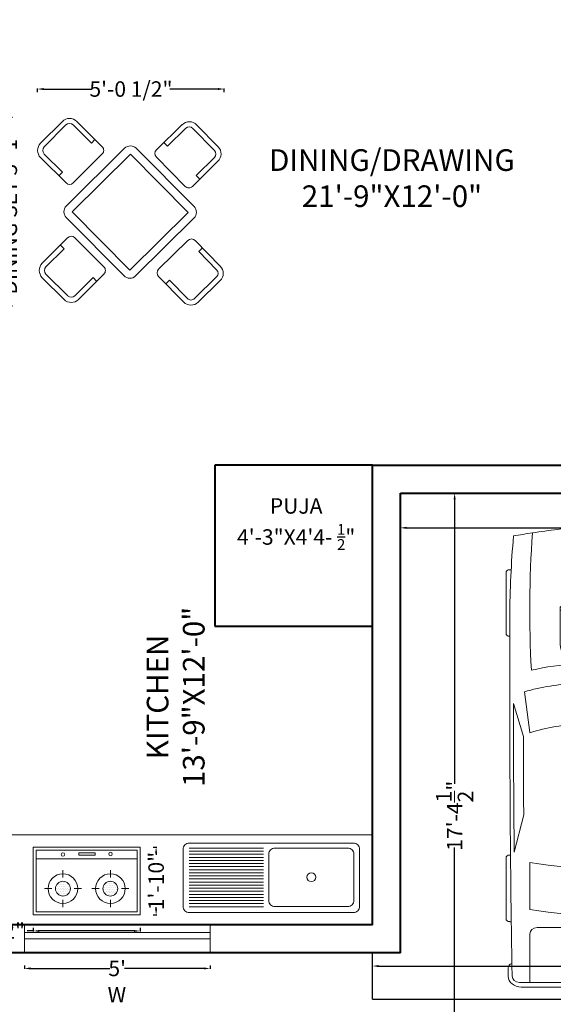
# Model space of a CAD drawing. Units: inches. Extents: x -231 to 349, y -511 to 252.
# Tile 3 of 6: x -36 to 136, y -351 to -33. Entities that reach past the tile are written whole.
import ezdxf

# ---------------------------------------------------------------- set-up
doc = ezdxf.new("R2010")
doc.units = ezdxf.units.IN
doc.header["$MEASUREMENT"] = 0
for name, color, linetype, lineweight in [('A-ANNO-DIMS', 7, 'Continuous', 18), ('A-ANNO-TEXT', 7, 'Continuous', 18), ('A-AREA-IDEN', 7, 'Continuous', 25), ('A-EQPM', 8, 'Continuous', 18), ('A-FLOR', 7, 'Continuous', 25), ('A-FLOR-CASE', 30, 'Continuous', 20), ('A-FLOR-FIXT', 8, 'Continuous', 18), ('A-FLOR-FIXT-PATT', 8, 'Continuous', 13), ('A-FURN', 8, 'Continuous', 18), ('A-GLAZ', 177, 'Continuous', 20), ('A-WALL', 7, 'Continuous', 40), ('C-PARK-VEHI', 8, 'Continuous', 13)]:
    doc.layers.add(name, color=color, linetype=linetype, lineweight=lineweight)
doc.styles.get("Standard").update_dxf_attribs({"font": 'arial.ttf'})
doc.dimstyles.get("Standard").update_dxf_attribs({"dimtxt": 5, "dimasz": 2, "dimexe": 0.18, "dimexo": 0.0625, "dimgap": 0.09, "dimtad": 0, "dimzin": 0, "dimdsep": 46, "dimlunit": 4, "dimtxsty": 'Standard', "dimcen": 0.09, "dimadec": 0, "dimazin": 0, "dimtfac": 1, "dimtofl": 0, "dimtmove": 0, "dimatfit": 3, "dimfxl": 1, "dimfxlon": 1, "dimtolj": 1, "dimtzin": 0, "dimarcsym": 0})

# ---------------------------------------------------------------- blocks, each defined once
blk = doc.blocks.new('*U7')
for p, q in [((21.1, 37.41), (21.1, 36.83)), ((46.55, 38.89), (22.35, 38.89)), ((47.8, 37.39), (47.8, 37.41)), ((87.99, 31.87), (74.76, 35.92)), ((134.31, 35.6), (119.29, 31.78)), ((135.45, 37.07), (135.45, 37.41)), ((136.7, 38.89), (160.9, 38.89)), ((162.15, 37.41), (162.15, 36.77)), ((186.47, -33.5), (186.47, 33.5)), ((188.4, -32.76), (188.4, 32.76)), ((70.03, 31.54), (86.41, 29.35)), ((138.42, 29.35), (157.25, 29.35)), ((186.47, 29.35), (167.01, 29.35)), ((164.52, 26.39), (164.52, -26.39)), ((32.27, 11.63), (36.13, 17.17)), ((36.13, 17.17), (50.94, 17.17)), ((29.77, 9.51), (51.68, 9.51)), ((32.12, 9.51), (32.12, 11.15)), ((58.92, -10.77), (58.92, 10.77)), ((66.55, -10.53), (66.55, 10.53)), ((82.74, 8.5), (82.74, -8.5)), ((186.47, -10.53), (186.47, 10.53)), ((3.27, 6.13), (0.1, 0.41)), ((0, 0), (51.68, 0)), ((0.1, -0.41), (3.27, -6.13)), ((29.77, -9.51), (51.68, -9.51)), ((32.12, -9.51), (32.12, -11.15)), ((32.27, -11.63), (36.13, -17.17)), ((36.13, -17.17), (50.94, -17.17)), ((86.41, -29.35), (70.03, -31.54)), ((157.25, -29.35), (138.42, -29.35)), ((167.01, -29.35), (186.47, -29.35)), ((87.99, -31.87), (74.76, -35.92)), ((134.31, -35.6), (119.29, -31.78)), ((21.1, -37.41), (21.1, -36.83)), ((46.55, -38.89), (22.35, -38.89)), ((47.8, -37.39), (47.8, -37.41)), ((135.45, -37.07), (135.45, -37.41)), ((136.7, -38.89), (160.9, -38.89)), ((162.15, -37.41), (162.15, -36.77))]:
    blk.add_line(p, q)
for centre, major_axis, ratio, start_param, end_param in [((266.03, -27.52), (0, 313.31), 0.842304, 1.367076, 1.39176), ((41.19, -490.86), (0, 528.23), 0.842304, 0.00281, 0.075598), ((22.35, 37.41), (0, -1.48), 0.842304, 3.141593, 4.712389), ((64.48, -10555.62), (0, 10593.03), 0.842304, -0.013397, 0.002797), ((46.55, 37.41), (0, 1.48), 0.842304, -1.570796, 0), ((64.48, -10555.62), (0, -10591.55), 0.842304, 3.133765, 3.140441), ((136.7, 37.41), (0, -1.48), 0.842304, 3.141593, 4.712389), ((160.9, 37.41), (0, 1.48), 0.842304, -1.570796, 0), ((180.63, 35.84), (0, 2.22), 0.842304, -0.013017, 1.249894), ((64.48, -10556.36), (0, 10595.31), 0.842304, -0.013397, -0.013017), ((183.98, 33.5), (0, -2.96), 0.842304, 1.570796, 3.128196), ((183.98, 32.76), (0, -5.25), 0.842304, 1.570796, 3.128196), ((95.79, -3666.35), (0, -3698.24), 0.842304, 3.134049, 3.144098), ((259.18, -27.52), (0, -305.3), 0.842304, 4.528606, 4.561838), ((37.47, -593.96), (0, -623.33), 0.842304, 3.096046, 3.200911), ((134.4, 5.39), (0, -89.78), 0.842304, 4.449482, 4.652344), ((135.29, 5.39), (0, 81.77), 0.842304, 1.245306, 1.50788), ((149.6, 2.8), (0, -79.58), 0.842304, 4.372215, 4.640744), ((17.08, 0), (0, 147.02), 0.842304, 4.511394, 4.913384), ((35.91, 0), (0, 147.02), 0.842304, 4.511394, 4.913384), ((167.01, 26.39), (0, 2.96), 0.842304, 0, 1.570796), ((-204.49, 52.4), (0, -250.96), 0.842304, 1.385369, 1.434372), ((13.04, 17.01), (0, 27.42), 0.842304, 4.435146, 4.718221), ((14.2, 17.01), (0, 27.42), 0.842304, 4.435146, 4.718221), ((50.79, 13.34), (6.34, -0.36), 0.603834, -1.395552, 1.581315), ((29.77, -46.66), (0, 56.17), 0.842304, 0, 0.590319), ((32.75, 11.15), (0, 0.74), 0.842304, 0.879714, 1.570796), ((0.62, 0), (0, -0.74), 0.842304, 4.131459, 5.293319), ((29.77, 46.66), (0, 56.17), 0.842304, 2.551274, 3.141593), ((-204.49, -52.4), (0, 250.96), 0.842304, -1.434372, -1.385369), ((32.75, -11.15), (0, -0.74), 0.842304, 4.712389, 5.403472), ((13.04, -17.01), (0, -27.42), 0.842304, 1.564964, 1.848039), ((14.2, -17.01), (0, -27.42), 0.842304, 1.564964, 1.848039), ((134.4, -5.39), (0, -89.78), 0.842304, -1.510751, -1.307889), ((135.29, -5.39), (0, -81.77), 0.842304, -1.50788, -1.245306), ((149.6, -2.8), (0, -79.58), 0.842304, -1.499151, -1.230623), ((259.18, 27.52), (0, 305.3), 0.842304, 1.721348, 1.754579), ((167.01, -26.39), (0, -2.96), 0.842304, 4.712389, 6.283185), ((266.03, 27.52), (0, 313.31), 0.842304, 1.749832, 1.774517), ((37.47, 593.96), (0, -623.33), 0.842304, -0.059319, 0.045547), ((95.79, 3666.35), (0, -3698.24), 0.842304, -0.002505, 0.007544), ((183.98, -33.5), (0, 2.96), 0.842304, 3.15499, 4.712389), ((183.98, -32.76), (0, -5.25), 0.842304, 0.013397, 1.570796), ((41.19, 490.86), (0, -528.23), 0.842304, -0.075598, -0.00281), ((22.35, -37.41), (0, 1.48), 0.842304, 1.570796, 3.141593), ((64.48, 10555.62), (0, 10593.03), 0.842304, 3.138796, 3.15499), ((46.55, -37.41), (0, -1.48), 0.842304, 0, 1.570796), ((64.48, 10555.62), (0, -10591.55), 0.842304, 0.001152, 0.007828), ((136.7, -37.41), (0, -1.48), 0.842304, -1.570796, 0), ((160.9, -37.41), (0, 1.48), 0.842304, 3.141593, 4.712389), ((180.63, -35.84), (0, -2.22), 0.842304, -1.249894, 0.013017), ((64.48, 10556.36), (0, 10595.31), 0.842304, 3.15461, 3.15499)]:
    blk.add_ellipse(centre, major_axis=major_axis, ratio=ratio, start_param=start_param, end_param=end_param)
at = {"extrusion": (0, 0, -1)}
blk.add_ellipse((50.79, -13.34), major_axis=(6.34, 0.36), ratio=0.603834, start_param=-1.395552, end_param=1.581315, dxfattribs=at)
blk = doc.blocks.new('A$C475E21CF')
for p, q in [((0, 444.5), (0, 0)), ((0, 444.5), (699.9, 444.5)), ((19.4, 425), (19.4, 19.4)), ((19.4, 425), (680.5, 425)), ((194.5, 393.9), (194.5, 345.2)), ((505.4, 393.9), (505.4, 345.2)), ((680.5, 425), (680.5, 19.4)), ((699.9, 444.5), (699.9, 0)), ((72.9, 272.3), (121.6, 272.3)), ((148.7, 264.1), (148.7, 264.1)), ((154.8, 276.2), (154.8, 276.2)), ((160.9, 288.4), (160.9, 288.4)), ((160.9, 264.1), (160.9, 264.1)), ((166.9, 300.5), (166.9, 300.5)), ((166.9, 276.2), (166.9, 276.2)), ((173, 288.4), (173, 288.4)), ((173, 264.1), (173, 264.1)), ((179.1, 300.5), (179.1, 300.5)), ((179.1, 276.2), (179.1, 276.2)), ((185.2, 312.7), (185.2, 312.7)), ((185.2, 288.4), (185.2, 288.4)), ((185.2, 264.1), (185.2, 264.1)), ((191.2, 300.5), (191.2, 300.5)), ((191.2, 276.2), (191.2, 276.2)), ((197.3, 312.7), (197.3, 312.7)), ((197.3, 288.4), (197.3, 288.4)), ((197.3, 264.1), (197.3, 264.1)), ((203.4, 300.5), (203.4, 300.5)), ((203.4, 276.2), (203.4, 276.2)), ((209.5, 312.7), (209.5, 312.7)), ((209.5, 288.4), (209.5, 288.4)), ((209.5, 264.1), (209.5, 264.1)), ((215.6, 300.5), (215.6, 300.5)), ((215.6, 276.2), (215.6, 276.2)), ((221.6, 288.4), (221.6, 288.4)), ((221.6, 264.1), (221.6, 264.1)), ((227.7, 300.5), (227.7, 300.5)), ((227.7, 276.2), (227.7, 276.2)), ((233.8, 288.4), (233.8, 288.4)), ((233.8, 264.1), (233.8, 264.1)), ((239.9, 276.2), (239.9, 276.2)), ((267.4, 272.3), (316, 272.3)), ((383.9, 272.3), (432.5, 272.3)), ((462, 268), (462, 268)), ((468, 280.2), (468, 280.2)), ((474.1, 292.3), (474.1, 292.3)), ((474.1, 268), (474.1, 268)), ((480.2, 304.5), (480.2, 304.5)), ((480.2, 280.2), (480.2, 280.2)), ((486.3, 292.3), (486.3, 292.3)), ((486.3, 268), (486.3, 268)), ((492.3, 304.5), (492.3, 304.5)), ((492.3, 280.2), (492.3, 280.2)), ((498.4, 316.6), (498.4, 316.6)), ((498.4, 292.3), (498.4, 292.3)), ((498.4, 268), (498.4, 268)), ((504.5, 304.5), (504.5, 304.5)), ((504.5, 280.2), (504.5, 280.2)), ((510.6, 316.6), (510.6, 316.6)), ((510.6, 292.3), (510.6, 292.3)), ((510.6, 268), (510.6, 268)), ((516.7, 304.5), (516.7, 304.5)), ((516.7, 280.2), (516.7, 280.2)), ((522.7, 316.6), (522.7, 316.6)), ((522.7, 292.3), (522.7, 292.3)), ((522.7, 268), (522.7, 268)), ((528.8, 304.5), (528.8, 304.5)), ((528.8, 280.2), (528.8, 280.2)), ((534.9, 292.3), (534.9, 292.3)), ((534.9, 268), (534.9, 268)), ((541, 304.5), (541, 304.5)), ((541, 280.2), (541, 280.2)), ((547, 292.3), (547, 292.3)), ((547, 268), (547, 268)), ((553.1, 280.2), (553.1, 280.2)), ((578.4, 272.3), (627, 272.3)), ((154.8, 251.9), (154.8, 251.9)), ((160.9, 239.8), (160.9, 239.8)), ((166.9, 251.9), (166.9, 251.9)), ((173, 239.8), (173, 239.8)), ((179.1, 251.9), (179.1, 251.9)), ((179.1, 227.6), (179.1, 227.6)), ((185.2, 239.8), (185.2, 239.8)), ((191.2, 251.9), (191.2, 251.9)), ((191.2, 227.6), (191.2, 227.6)), ((194.5, 199.4), (194.5, 150.8)), ((197.3, 239.8), (197.3, 239.8)), ((203.4, 251.9), (203.4, 251.9)), ((203.4, 227.6), (203.4, 227.6)), ((209.5, 239.8), (209.5, 239.8)), ((215.6, 251.9), (215.6, 251.9)), ((215.6, 227.6), (215.6, 227.6)), ((221.6, 239.8), (221.6, 239.8)), ((227.7, 251.9), (227.7, 251.9)), ((233.8, 239.8), (233.8, 239.8)), ((239.9, 251.9), (239.9, 251.9)), ((468, 255.9), (468, 255.9)), ((474.1, 243.7), (474.1, 243.7)), ((480.2, 255.9), (480.2, 255.9)), ((486.3, 243.7), (486.3, 243.7)), ((492.3, 255.9), (492.3, 255.9)), ((492.3, 231.5), (492.3, 231.5)), ((498.4, 243.7), (498.4, 243.7)), ((504.5, 255.9), (504.5, 255.9)), ((504.5, 231.5), (504.5, 231.5)), ((505.4, 199.4), (505.4, 150.8)), ((510.6, 243.7), (510.6, 243.7)), ((516.7, 255.9), (516.7, 255.9)), ((516.7, 231.5), (516.7, 231.5)), ((522.7, 243.7), (522.7, 243.7)), ((528.8, 255.9), (528.8, 255.9)), ((528.8, 231.5), (528.8, 231.5)), ((534.9, 243.7), (534.9, 243.7)), ((541, 255.9), (541, 255.9)), ((547, 243.7), (547, 243.7)), ((553.1, 255.9), (553.1, 255.9)), ((19.4, 77.8), (680.5, 77.8)), ((0, 0), (699.9, 0)), ((19.4, 19.4), (680.5, 19.4)), ((293.4, 51.9), (400.6, 51.9)), ((293.4, 36.5), (293.4, 51.9)), ((400.6, 36.5), (293.4, 36.5)), ((400.6, 51.9), (400.6, 36.5))]:
    blk.add_line(p, q)
for centre, radius in [((194.5, 272.3), 97.2), ((505.4, 272.3), 97.2), ((194.5, 272.3), 48.6), ((505.4, 272.3), 48.6), ((193.9, 45.1), 11.7), ((505.2, 48.5), 11.7)]:
    blk.add_circle(centre, radius)
blk = doc.blocks.new('*D11')
at = {"layer": 'A-ANNO-DIMS', "color": 0, "lineweight": -2, "transparency": 16777216}
for p, q in [((77.92, -339.94), (77.92, -338.76)), ((79.92, -338.94), (154.98, -338.94)), ((246.92, -338.94), (171.86, -338.94)), ((248.92, -339.94), (248.92, -338.76))]:
    blk.add_line(p, q, dxfattribs=at)
at = {"layer": 'A-ANNO-DIMS', "color": 0, "transparency": 16777216}
for points in [[(79.92, -338.61), (79.92, -339.28), (77.92, -338.94)], [(246.92, -338.61), (246.92, -339.28), (248.92, -338.94)]]:
    blk.add_solid(points, dxfattribs=at)
at = {"layer": 'Defpoints', "color": 0, "transparency": 16777216}
for p in [(248.92, -338.94), (77.92, -342.12), (248.92, -342.12)]:
    blk.add_point(p, dxfattribs=at)
at = {"layer": 'A-ANNO-DIMS', "color": 0, "transparency": 16777216, "insert": (163.42, -338.94), "char_height": 5, "attachment_point": 5}
blk.add_mtext('\\A1;14\'-3"', dxfattribs=at)
blk = doc.blocks.new('*D21')
at = {"layer": 'A-ANNO-DIMS', "color": 0, "lineweight": -2, "transparency": 16777216}
for p, q in [((-34.58, -338.71), (-34.58, -339.89)), ((-32.58, -339.71), (-6.97, -339.71)), ((23.42, -339.71), (-2.19, -339.71)), ((25.42, -338.71), (25.42, -339.89))]:
    blk.add_line(p, q, dxfattribs=at)
at = {"layer": 'A-ANNO-DIMS', "color": 0, "transparency": 16777216}
for points in [[(-32.58, -339.38), (-32.58, -340.05), (-34.58, -339.71)], [(23.42, -339.38), (23.42, -340.05), (25.42, -339.71)]]:
    blk.add_solid(points, dxfattribs=at)
at = {"layer": 'Defpoints', "color": 0, "transparency": 16777216}
for p in [(-34.58, -334.62), (25.42, -334.62), (25.42, -339.71)]:
    blk.add_point(p, dxfattribs=at)
at = {"layer": 'A-ANNO-DIMS', "color": 0, "transparency": 16777216, "insert": (-4.58, -339.71), "char_height": 5, "attachment_point": 5}
blk.add_mtext("\\A1;5'", dxfattribs=at)
blk = doc.blocks.new('A$C14754BF6')
for p, q in [((0.0258, 1.5763), (0.2378, 1.7886)), ((0.0612, 1.541), (0.2732, 1.7533)), ((0.5208, 1.5767), (0.3439, 1.7533)), ((0.6269, 1.5414), (0.3792, 1.7887)), ((1.1555, 1.5114), (1.4054, 1.7564)), ((1.7568, 1.5407), (1.5468, 1.7549)), ((1.2619, 1.5457), (1.4404, 1.7207)), ((1.7211, 1.5057), (1.5111, 1.7199)), ((0.5208, 1.5767), (0.5561, 1.6121)), ((1.2619, 1.5457), (1.2269, 1.5814)), ((0.2382, 1.2936), (0.0613, 1.4703)), ((0.8454, 1.5266), (0.2771, 0.9635)), ((0.9017, 1.4697), (0.3334, 0.9067)), ((0.3444, 1.1876), (0.627, 1.4707)), ((0.9017, 1.4697), (1.4647, 0.9014)), ((0.9585, 1.526), (1.5216, 0.9577)), ((1.4347, 1.155), (1.1547, 1.4407)), ((0.2736, 1.1876), (0.026, 1.4349)), ((1.5054, 1.1543), (1.7554, 1.3993)), ((1.5418, 1.26), (1.7204, 1.435)), ((0.2029, 1.2582), (0.2382, 1.2936)), ((1.5768, 1.2243), (1.5418, 1.26)), ((0.3334, 0.9067), (0.8964, 0.3384)), ((1.4647, 0.9014), (0.8964, 0.3384)), ((0.2766, 0.8504), (0.8396, 0.2821)), ((1.521, 0.8446), (0.9527, 0.2815)), ((0.2893, 0.6533), (0.0421, 0.4056)), ((0.2541, 0.5472), (0.2187, 0.5826)), ((0.6431, 0.3708), (0.3601, 0.6534)), ((1.1767, 0.3475), (1.4623, 0.6275)), ((1.533, 0.6268), (1.778, 0.3768)), ((0.2541, 0.5472), (0.0774, 0.3703)), ((1.5673, 0.5204), (1.603, 0.5554)), ((1.5673, 0.5204), (1.7423, 0.3418)), ((0.2898, 0.0876), (0.0775, 0.2996)), ((0.6432, 0.3), (0.3959, 0.0524)), ((0.2545, 0.0523), (0.0422, 0.2642)), ((0.5371, 0.2646), (0.3605, 0.0877)), ((0.5725, 0.2293), (0.5371, 0.2646)), ((1.1759, 0.2768), (1.4209, 0.0269)), ((1.2459, 0.2054), (1.2816, 0.2404)), ((1.2816, 0.2404), (1.4566, 0.0619)), ((1.5273, 0.0611), (1.7416, 0.2711)), ((1.5623, 0.0254), (1.7766, 0.2354))]:
    blk.add_line(p, q)
for centre, radius, start, end in [((0.3086, 1.7179), 0.1, 45.0454, 135.0454), ((0.3086, 1.7179), 0.05, 45.0454, 135.0454), ((1.4754, 1.6849), 0.1, 44.42077, 134.42077), ((1.4754, 1.6849), 0.05, 44.42077, 134.42077), ((0.0966, 1.5056), 0.1, 135.0454, 225.0454), ((0.0966, 1.5056), 0.05, 135.0454, 225.0454), ((0.5916, 1.506), 0.05, 315.0454, 45.0454), ((0.9017, 1.4697), 0.08, 44.73309, 134.73309), ((1.6854, 1.4707), 0.1, 314.42077, 44.42077), ((1.1905, 1.4757), 0.05, 134.42077, 224.42077), ((1.6854, 1.4707), 0.05, 314.42077, 44.42077), ((0.309, 1.223), 0.05, 225.0454, 315.0454), ((1.4704, 1.19), 0.05, 224.42077, 314.42077), ((0.3334, 0.9067), 0.08, 134.73309, 224.73309), ((1.4647, 0.9014), 0.08, 314.73309, 44.73309), ((0.3247, 0.618), 0.05, 45.0454, 135.0454), ((1.4973, 0.5918), 0.05, 44.42077, 134.42077), ((0.1128, 0.335), 0.1, 135.0454, 225.0454), ((0.1128, 0.335), 0.05, 135.0454, 225.0454), ((0.6078, 0.3354), 0.05, 315.0454, 45.0454), ((1.2117, 0.3118), 0.05, 134.42077, 224.42077), ((1.7066, 0.3068), 0.05, 314.42077, 44.42077), ((1.7066, 0.3068), 0.1, 314.42077, 44.42077), ((0.8964, 0.3384), 0.08, 224.73309, 314.73309), ((0.3251, 0.123), 0.1, 225.0454, 315.0454), ((0.3251, 0.123), 0.05, 225.0454, 315.0454), ((1.4923, 0.0968), 0.1, 224.42077, 314.42077), ((1.4923, 0.0968), 0.05, 224.42077, 314.42077)]:
    blk.add_arc(centre, radius, start, end)
blk = doc.blocks.new('*D26')
at = {"layer": 'A-ANNO-DIMS', "color": 0, "lineweight": -2, "transparency": 16777216}
for p, q in [((105.45, -186.12), (104.27, -186.12)), ((104.45, -188.12), (104.45, -280.1)), ((104.45, -392.62), (104.45, -300.64)), ((105.45, -394.62), (104.27, -394.62))]:
    blk.add_line(p, q, dxfattribs=at)
at = {"layer": 'A-ANNO-DIMS', "color": 0, "transparency": 16777216}
for points in [[(104.12, -188.12), (104.79, -188.12), (104.45, -186.12)], [(104.12, -392.62), (104.79, -392.62), (104.45, -394.62)]]:
    blk.add_solid(points, dxfattribs=at)
at = {"layer": 'Defpoints', "color": 0, "transparency": 16777216}
for p in [(104.45, -186.12), (115.6, -186.12), (115.6, -394.62)]:
    blk.add_point(p, dxfattribs=at)
at = {"layer": 'A-ANNO-DIMS', "color": 0, "transparency": 16777216, "insert": (104.45, -290.37), "char_height": 5, "attachment_point": 5, "rotation": 90}
blk.add_mtext('\\A1;17\'-4{\\H1x;\\S1/2;}"', dxfattribs=at)
blk = doc.blocks.new('*D27')
at = {"layer": 'A-ANNO-DIMS', "color": 0, "lineweight": -2, "transparency": 16777216}
for p, q in [((86.92, -198.32), (86.92, -197.14)), ((269.92, -198.32), (269.92, -197.14)), ((88.92, -197.32), (169.98, -197.32)), ((267.92, -197.32), (186.86, -197.32))]:
    blk.add_line(p, q, dxfattribs=at)
at = {"layer": 'A-ANNO-DIMS', "color": 0, "transparency": 16777216}
for points in [[(88.92, -196.99), (88.92, -197.66), (86.92, -197.32)], [(267.92, -196.99), (267.92, -197.66), (269.92, -197.32)]]:
    blk.add_solid(points, dxfattribs=at)
at = {"layer": 'Defpoints', "color": 0, "transparency": 16777216}
for p in [(269.92, -197.32), (86.92, -211.86), (269.92, -211.86)]:
    blk.add_point(p, dxfattribs=at)
at = {"layer": 'A-ANNO-DIMS', "color": 0, "transparency": 16777216, "insert": (178.42, -197.32), "char_height": 5, "attachment_point": 5}
blk.add_mtext('\\A1;15\'-3"', dxfattribs=at)
blk = doc.blocks.new('*D38')
at = {"layer": 'A-ANNO-DIMS', "color": 0, "lineweight": -2, "transparency": 16777216}
for p, q in [((-31.7, -327.6), (-33.7, -327.6)), ((-31.7, -326.6), (-31.7, -327.78)), ((0.82, -327.6), (-29.7, -327.6)), ((2.82, -326.6), (2.82, -327.78))]:
    blk.add_line(p, q, dxfattribs=at)
at = {"layer": 'A-ANNO-DIMS', "color": 0, "transparency": 16777216}
for points in [[(-29.7, -327.27), (-29.7, -327.94), (-31.7, -327.6)], [(0.82, -327.27), (0.82, -327.94), (2.82, -327.6)]]:
    blk.add_solid(points, dxfattribs=at)
at = {"layer": 'Defpoints', "color": 0, "transparency": 16777216}
for p in [(-31.7, -322.43), (2.82, -322.43), (-31.7, -327.6)]:
    blk.add_point(p, dxfattribs=at)
at = {"layer": 'A-ANNO-DIMS', "color": 0, "transparency": 16777216, "insert": (-66.61, -327.6), "char_height": 5, "attachment_point": 5}
blk.add_mtext('\\A1;COOKTOP 2\'-10 1/2"', dxfattribs=at)
blk = doc.blocks.new('*D39')
at = {"layer": 'A-ANNO-DIMS', "color": 0, "lineweight": -2, "transparency": 16777216}
for p, q in [((7, -300.5), (8.18, -300.5)), ((8, -302.5), (8, -303.02)), ((8, -320.43), (8, -319.91)), ((7, -322.43), (8.18, -322.43))]:
    blk.add_line(p, q, dxfattribs=at)
at = {"layer": 'A-ANNO-DIMS', "color": 0, "transparency": 16777216}
for points in [[(7.66, -302.5), (8.33, -302.5), (8, -300.5)], [(7.66, -320.43), (8.33, -320.43), (8, -322.43)]]:
    blk.add_solid(points, dxfattribs=at)
at = {"layer": 'Defpoints', "color": 0, "transparency": 16777216}
for p in [(2.82, -300.5), (2.82, -322.43), (8, -322.43)]:
    blk.add_point(p, dxfattribs=at)
at = {"layer": 'A-ANNO-DIMS', "color": 0, "transparency": 16777216, "insert": (8, -311.46), "char_height": 5, "attachment_point": 5, "rotation": 90}
blk.add_mtext('\\A1;1\'-10"', dxfattribs=at)
blk = doc.blocks.new('*D40')
at = {"layer": 'A-ANNO-DIMS', "color": 0, "lineweight": -2, "transparency": 16777216}
for p, q in [((-38.45, -64.68), (-39.63, -64.68)), ((-39.45, -66.68), (-39.45, -67.62)), ((-39.45, -123.69), (-39.45, -122.75)), ((-38.45, -125.69), (-39.63, -125.69))]:
    blk.add_line(p, q, dxfattribs=at)
at = {"layer": 'A-ANNO-DIMS', "color": 0, "transparency": 16777216}
for points in [[(-39.78, -66.68), (-39.12, -66.68), (-39.45, -64.68)], [(-39.78, -123.69), (-39.12, -123.69), (-39.45, -125.69)]]:
    blk.add_solid(points, dxfattribs=at)
at = {"layer": 'Defpoints', "color": 0, "transparency": 16777216}
for p in [(-39.45, -64.68), (-30.3, -64.68), (-30.3, -125.69)]:
    blk.add_point(p, dxfattribs=at)
at = {"layer": 'A-ANNO-DIMS', "color": 0, "transparency": 16777216, "insert": (-39.45, -95.19), "char_height": 5, "attachment_point": 5, "rotation": 90}
blk.add_mtext('\\A1;DINING SET 5\'-1"', dxfattribs=at)
blk = doc.blocks.new('*D41')
at = {"layer": 'A-ANNO-DIMS', "color": 0, "lineweight": -2, "transparency": 16777216}
for p, q in [((-30.3, -56.53), (-30.3, -55.35)), ((-28.3, -55.53), (-12.7, -55.53)), ((28.03, -55.53), (12.43, -55.53)), ((30.03, -56.53), (30.03, -55.35))]:
    blk.add_line(p, q, dxfattribs=at)
at = {"layer": 'A-ANNO-DIMS', "color": 0, "transparency": 16777216}
for points in [[(-28.3, -55.19), (-28.3, -55.86), (-30.3, -55.53)], [(28.03, -55.19), (28.03, -55.86), (30.03, -55.53)]]:
    blk.add_solid(points, dxfattribs=at)
at = {"layer": 'Defpoints', "color": 0, "transparency": 16777216}
for p in [(30.03, -55.53), (-30.3, -64.68), (30.03, -64.68)]:
    blk.add_point(p, dxfattribs=at)
at = {"layer": 'A-ANNO-DIMS', "color": 0, "transparency": 16777216, "insert": (-0.13, -55.53), "char_height": 5, "attachment_point": 5}
blk.add_mtext('\\A1;5\'-0 1/2"', dxfattribs=at)
blk = doc.blocks.new('*D51')
at = {"layer": 'A-ANNO-DIMS', "color": 0, "lineweight": -2, "transparency": 16777216}
for p, q in [((26.42, -489.55), (24.42, -489.55)), ((28.42, -488.55), (28.42, -489.73)), ((32.24, -488.55), (32.24, -489.73)), ((34.24, -489.55), (36.24, -489.55))]:
    blk.add_line(p, q, dxfattribs=at)
at = {"layer": 'A-ANNO-DIMS', "color": 0, "transparency": 16777216}
for points in [[(26.42, -489.21), (26.42, -489.88), (28.42, -489.55)], [(34.24, -489.21), (34.24, -489.88), (32.24, -489.55)]]:
    blk.add_solid(points, dxfattribs=at)
at = {"layer": 'Defpoints', "color": 0, "transparency": 16777216}
for p in [(28.42, 133.38), (32.24, 133.38), (32.24, -489.55)]:
    blk.add_point(p, dxfattribs=at)
at = {"layer": 'A-ANNO-DIMS', "color": 0, "transparency": 16777216, "insert": (42.97, -489.55), "char_height": 5, "attachment_point": 5}
blk.add_mtext('\\A1;0\'-4"', dxfattribs=at)
blk = doc.blocks.new('*D56')
at = {"layer": 'A-ANNO-DIMS', "color": 0, "lineweight": -2, "transparency": 16777216}
for p, q in [((-96.08, -488.55), (-96.08, -489.73)), ((-94.08, -489.55), (-77.89, -489.55)), ((-36.58, -489.55), (-52.77, -489.55)), ((-34.58, -488.55), (-34.58, -489.73))]:
    blk.add_line(p, q, dxfattribs=at)
at = {"layer": 'A-ANNO-DIMS', "color": 0, "transparency": 16777216}
for points in [[(-94.08, -489.21), (-94.08, -489.88), (-96.08, -489.55)], [(-36.58, -489.21), (-36.58, -489.88), (-34.58, -489.55)]]:
    blk.add_solid(points, dxfattribs=at)
at = {"layer": 'Defpoints', "color": 0, "transparency": 16777216}
for p in [(-96.08, -334.62), (-34.58, -334.62), (-34.58, -489.55)]:
    blk.add_point(p, dxfattribs=at)
at = {"layer": 'A-ANNO-DIMS', "color": 0, "transparency": 16777216, "insert": (-65.33, -489.55), "char_height": 5, "attachment_point": 5}
blk.add_mtext('\\A1;5\'-1 1/2"', dxfattribs=at)
blk = doc.blocks.new('*D58')
at = {"layer": 'A-ANNO-DIMS', "color": 0, "lineweight": -2, "transparency": 16777216}
for p, q in [((-18.2, -488.55), (-18.2, -489.73)), ((-16.2, -489.55), (-6.93, -489.55)), ((15.8, -489.55), (6.54, -489.55)), ((17.8, -488.55), (17.8, -489.73))]:
    blk.add_line(p, q, dxfattribs=at)
at = {"layer": 'A-ANNO-DIMS', "color": 0, "transparency": 16777216}
for points in [[(-16.2, -489.21), (-16.2, -489.88), (-18.2, -489.55)], [(15.8, -489.21), (15.8, -489.88), (17.8, -489.55)]]:
    blk.add_solid(points, dxfattribs=at)
at = {"layer": 'Defpoints', "color": 0, "transparency": 16777216}
for p in [(-18.2, -33.12), (17.8, -33.12), (17.8, -489.55)]:
    blk.add_point(p, dxfattribs=at)
at = {"layer": 'A-ANNO-DIMS', "color": 0, "transparency": 16777216, "insert": (-0.2, -489.55), "char_height": 5, "attachment_point": 5}
blk.add_mtext('\\A1;3\'-0"', dxfattribs=at)
blk = doc.blocks.new('*D59')
at = {"layer": 'A-ANNO-DIMS', "color": 0, "lineweight": -2, "transparency": 16777216}
for p, q in [((17.8, -488.55), (17.8, -489.73)), ((19.8, -489.55), (21.92, -489.55)), ((23.92, -488.55), (23.92, -489.73)), ((23.92, -489.55), (25.92, -489.55))]:
    blk.add_line(p, q, dxfattribs=at)
at = {"layer": 'A-ANNO-DIMS', "color": 0, "transparency": 16777216}
for points in [[(19.8, -489.21), (19.8, -489.88), (17.8, -489.55)], [(21.92, -489.21), (21.92, -489.88), (23.92, -489.55)]]:
    blk.add_solid(points, dxfattribs=at)
at = {"layer": 'Defpoints', "color": 0, "transparency": 16777216}
for p in [(17.8, -28.62), (23.92, -33.12), (23.92, -489.55)]:
    blk.add_point(p, dxfattribs=at)
at = {"layer": 'A-ANNO-DIMS', "color": 0, "transparency": 16777216, "insert": (32.66, -489.55), "char_height": 5, "attachment_point": 5}
blk.add_mtext('\\A1;0\'-6"', dxfattribs=at)
blk = doc.blocks.new('*D60')
at = {"layer": 'A-ANNO-DIMS', "color": 0, "lineweight": -2, "transparency": 16777216}
for p, q in [((82.42, -488.55), (82.42, -489.73)), ((84.42, -489.55), (84.92, -489.55)), ((86.92, -488.55), (86.92, -489.73)), ((86.92, -489.55), (88.92, -489.55))]:
    blk.add_line(p, q, dxfattribs=at)
at = {"layer": 'A-ANNO-DIMS', "color": 0, "transparency": 16777216}
for points in [[(84.42, -489.21), (84.42, -489.88), (82.42, -489.55)], [(84.92, -489.21), (84.92, -489.88), (86.92, -489.55)]]:
    blk.add_solid(points, dxfattribs=at)
at = {"layer": 'Defpoints', "color": 0, "transparency": 16777216}
for p in [(82.42, -33.12), (86.92, -33.12), (86.92, -489.55)]:
    blk.add_point(p, dxfattribs=at)
at = {"layer": 'A-ANNO-DIMS', "color": 0, "transparency": 16777216, "insert": (101.48, -489.55), "char_height": 5, "attachment_point": 5}
blk.add_mtext('\\A1;0\'-4 1/2"', dxfattribs=at)
blk = doc.blocks.new('*D64')
at = {"layer": 'A-ANNO-DIMS', "color": 0, "lineweight": -2, "transparency": 16777216}
for p, q in [((333.44, -16.46), (334.62, -16.46)), ((334.44, -18.46), (334.44, -26.62)), ((333.44, -28.62), (334.62, -28.62)), ((334.44, -28.62), (334.44, -30.62))]:
    blk.add_line(p, q, dxfattribs=at)
at = {"layer": 'A-ANNO-DIMS', "color": 0, "transparency": 16777216}
for points in [[(334.11, -18.46), (334.78, -18.46), (334.44, -16.46)], [(334.11, -26.62), (334.78, -26.62), (334.44, -28.62)]]:
    blk.add_solid(points, dxfattribs=at)
at = {"layer": 'Defpoints', "color": 0, "transparency": 16777216}
for p in [(82.42, -16.46), (82.42, -28.62), (334.44, -28.62)]:
    blk.add_point(p, dxfattribs=at)
at = {"layer": 'A-ANNO-DIMS', "color": 0, "transparency": 16777216, "insert": (334.44, -37.12), "char_height": 5, "attachment_point": 5, "rotation": 90}
blk.add_mtext('\\A1;1\'-0"', dxfattribs=at)
blk = doc.blocks.new('*D67')
at = {"layer": 'A-ANNO-DIMS', "color": 0, "lineweight": -2, "transparency": 16777216}
for p, q in [((333.44, -141.12), (334.62, -141.12)), ((334.44, -143.12), (334.44, -152.39)), ((334.44, -175.12), (334.44, -165.85)), ((333.44, -177.12), (334.62, -177.12))]:
    blk.add_line(p, q, dxfattribs=at)
at = {"layer": 'A-ANNO-DIMS', "color": 0, "transparency": 16777216}
for points in [[(334.11, -143.12), (334.78, -143.12), (334.44, -141.12)], [(334.11, -175.12), (334.78, -175.12), (334.44, -177.12)]]:
    blk.add_solid(points, dxfattribs=at)
at = {"layer": 'Defpoints', "color": 0, "transparency": 16777216}
for p in [(-36.08, -141.12), (334.44, -141.12), (-36.08, -177.12)]:
    blk.add_point(p, dxfattribs=at)
at = {"layer": 'A-ANNO-DIMS', "color": 0, "transparency": 16777216, "insert": (334.44, -159.12), "char_height": 5, "attachment_point": 5, "rotation": 90}
blk.add_mtext('\\A1;3\'-0"', dxfattribs=at)
blk = doc.blocks.new('*D68')
at = {"layer": 'A-ANNO-DIMS', "color": 0, "lineweight": -2, "transparency": 16777216}
for p, q in [((-48.08, 213.78), (-48.08, 214.96)), ((-46.08, 214.78), (-38.08, 214.78)), ((-36.08, 213.78), (-36.08, 214.96)), ((-36.08, 214.78), (-34.08, 214.78))]:
    blk.add_line(p, q, dxfattribs=at)
at = {"layer": 'A-ANNO-DIMS', "color": 0, "transparency": 16777216}
for points in [[(-46.08, 215.11), (-46.08, 214.45), (-48.08, 214.78)], [(-38.08, 215.11), (-38.08, 214.45), (-36.08, 214.78)]]:
    blk.add_solid(points, dxfattribs=at)
at = {"layer": 'Defpoints', "color": 0, "transparency": 16777216}
for p in [(-36.08, 214.78), (-48.08, -177.12), (-36.08, -177.12)]:
    blk.add_point(p, dxfattribs=at)
at = {"layer": 'A-ANNO-DIMS', "color": 0, "transparency": 16777216, "insert": (-27.58, 214.78), "char_height": 5, "attachment_point": 5}
blk.add_mtext('\\A1;1\'-0"', dxfattribs=at)

msp = doc.modelspace()

# ---------------------------------------------------------------- hatches: boundary and pattern name
at = {"layer": 'A-FLOR-FIXT-PATT'}
h = msp.add_hatch(dxfattribs=at)
h.set_pattern_fill('ANSI31', color=256, scale=7.96897, angle=-45, style=0)
h.paths.add_polyline_path([(18.665, -320.22), (42.705, -320.22), (42.705, -300.298), (18.665, -300.298)])

# ---------------------------------------------------------------- linework, layer by layer
at = {"layer": 'A-FLOR'}
for q in [(77.92, -334.62), (248.92, -349.62)]:
    msp.add_line((77.92, -349.62), q, dxfattribs=at)
at = {"layer": 'A-FLOR-CASE'}
msp.add_line((77.92, -296.522), (-55.326, -296.522), dxfattribs=at)
at = {"layer": 'A-FLOR-FIXT'}
for points in [[(18.732, -299.186), (71.722, -299.186, -0.4142136), (73.722, -301.186), (73.722, -319.668, -0.4142136), (71.722, -321.668), (18.732, -321.668, -0.4142136), (16.732, -319.668), (16.732, -301.186, -0.4142136)], [(69.897, -300.796), (46.421, -300.796, 0.4142136), (44.421, -302.796), (44.421, -317.722, 0.4142136), (46.421, -319.722), (69.897, -319.722, 0.4142136), (71.897, -317.722), (71.897, -302.796, 0.4142136)]]:
    msp.add_lwpolyline(points, format="xyb", close=True, dxfattribs=at)
msp.add_circle((58.159, -310.259), 1.409, dxfattribs=at)
at = {"layer": 'A-GLAZ'}
for p, q in [((-34.58, -325.62), (-34.58, -334.62)), ((25.42, -325.62), (25.42, -334.62)), ((-34.58, -328.12), (25.42, -328.12)), ((-34.58, -330.12), (25.42, -330.12))]:
    msp.add_line(p, q, dxfattribs=at)
at = {"layer": 'A-WALL'}
for p, q in [((77.92, -177.12), (26.92, -177.12)), ((26.92, -177.12), (26.92, -229.12)), ((77.92, -177.12), (158.708, -177.12)), ((77.92, -325.62), (77.92, -177.12)), ((86.92, -334.62), (86.92, -186.12)), ((86.92, -186.12), (233.92, -186.12)), ((26.92, -229.12), (77.92, -229.12)), ((77.92, -325.62), (-87.08, -325.62)), ((86.92, -334.62), (-96.08, -334.62))]:
    msp.add_line(p, q, dxfattribs=at)

# ---------------------------------------------------------------- block references
at = {"layer": 'A-EQPM', "xscale": 0.0493232478550035, "yscale": 0.0493232478550035, "zscale": 0.0493232478550035, "rotation": 180}
msp.add_blockref('A$C475E21CF', (2.818, -300.501), dxfattribs=at)
at = {"layer": 'A-FURN', "xscale": 33.14342024626885, "yscale": 33.14342024626885, "zscale": 33.14342024626885}
msp.add_blockref('A$C14754BF6', (-30.184, -125.255), dxfattribs=at)
at = {"layer": 'C-PARK-VEHI', "xscale": 0.806401405747885, "yscale": 0.806401405747885, "zscale": 0.806401405747885, "rotation": 270}
msp.add_blockref('*U7', (152.419, -193.841), dxfattribs=at)

# ---------------------------------------------------------------- texts
at = {"layer": 'A-ANNO-TEXT', "insert": (-7.674, -345.694), "char_height": 5, "attachment_point": 1}
msp.add_mtext_dynamic_manual_height_columns('\\A1;W', width=7.82759, gutter_width=1, heights=[0], dxfattribs=at)
at = {"layer": 'A-AREA-IDEN', "attachment_point": 1}
for s, insert, char_height in [('\\pxqc;DINING/DRAWING\\P21\'-9"X12\'-0"', (32.877, -74.989), 7), ('\\A1;\\pxqc;PUJA\\P4\'-3"X4\'4- {\\H0.7x;\\S1/2;}"', (1.919, -187.751), 5)]:
    msp.add_mtext_dynamic_manual_height_columns(s, width=102.65834, gutter_width=1, heights=[0], dxfattribs=dict(at, insert=insert, char_height=char_height))
at = {"layer": 'A-AREA-IDEN', "insert": (4.986, -303.296), "char_height": 7, "attachment_point": 1, "rotation": 90}
msp.add_mtext_dynamic_manual_height_columns('\\pxqc;KITCHEN\\P13\'-9"X12\'-0"', width=102.65834, gutter_width=1, heights=[0], dxfattribs=at)

# ---------------------------------------------------------------- dimensions: what is measured, and where the dimension line sits
at = {"layer": 'A-ANNO-DIMS'}
for base, p1, p2, override, picture, middle in [((-36.08, 214.78), (-48.08, -177.12), (-36.08, -177.12), {"dimdec": 1, "dimlfac": 1, "dimrnd": 0, "dimzin": 1, "dimdsep": 46, "dimlunit": 4, "dimfrac": 2}, '*D68', (-27.58, 214.78)), ((32.236, -489.548), (28.42, 133.38), (32.236, 133.38), {"dimdec": 1, "dimlfac": 1, "dimrnd": 0, "dimzin": 1, "dimdsep": 46, "dimlunit": 4, "dimfrac": 2}, '*D51', (42.971, -489.548)), ((23.92, -489.548), (17.803, -28.62), (23.92, -33.12), {"dimdec": 1, "dimlfac": 1, "dimrnd": 0, "dimzin": 1, "dimdsep": 46, "dimlunit": 4, "dimfrac": 2}, '*D59', (32.655, -489.548)), ((17.803, -489.548), (-18.197, -33.12), (17.803, -33.12), {"dimdec": 1, "dimlfac": 1, "dimrnd": 0, "dimzin": 1, "dimdsep": 46, "dimlunit": 4, "dimfrac": 2}, '*D58', (-0.197, -489.548)), ((86.92, -489.548), (82.42, -33.12), (86.92, -33.12), {"dimdec": 1, "dimlfac": 1, "dimrnd": 0, "dimzin": 1, "dimdsep": 46, "dimlunit": 4, "dimfrac": 2}, '*D60', (101.481, -489.548)), ((30.027, -55.526), (-30.297, -64.678), (30.027, -64.678), {"dimdec": 1, "dimlfac": 1, "dimrnd": 0, "dimzin": 1, "dimdsep": 46, "dimlunit": 4, "dimfrac": 2}, '*D41', (-0.135, -55.526)), ((269.92, -197.325), (86.92, -211.864), (269.92, -211.864), {"dimclrd": 0, "dimclre": 0, "dimclrt": 0}, '*D27', (178.42, -197.325)), ((-34.58, -489.548), (-96.08, -334.62), (-34.58, -334.62), {"dimdec": 1, "dimlfac": 1, "dimrnd": 0, "dimzin": 1, "dimdsep": 46, "dimlunit": 4, "dimfrac": 2}, '*D56', (-65.33, -489.548)), ((25.42, -339.714), (-34.58, -334.62), (25.42, -334.62), {"dimclrd": 0, "dimclre": 0, "dimclrt": 0}, '*D21', (-4.58, -339.714)), ((248.92, -338.944), (77.92, -342.12), (248.92, -342.12), {"dimclrd": 0, "dimclre": 0, "dimclrt": 0}, '*D11', (163.42, -338.944))]:
    dim = msp.add_linear_dim(base=base, p1=p1, p2=p2, dimstyle='Standard', override=override, dxfattribs=at)
    dim.commit()
    dim.dimension.update_dxf_attribs({"geometry": picture, "text_midpoint": middle})
for base, p1, p2, angle, override, picture, middle in [((334.442, -28.62), (82.42, -16.457), (82.42, -28.62), 90, {"dimdec": 1, "dimlfac": 1, "dimrnd": 0, "dimzin": 1, "dimdsep": 46, "dimlunit": 4, "dimfrac": 2}, '*D64', (334.442, -37.121)), ((334.442, -141.12), (-36.08, -177.12), (-36.08, -141.12), 90, {"dimdec": 1, "dimlfac": 1, "dimrnd": 0, "dimzin": 1, "dimdsep": 46, "dimlunit": 4, "dimfrac": 2}, '*D67', (334.442, -159.12)), ((104.455, -186.12), (115.598, -394.62), (115.598, -186.12), 90, {"dimclrd": 0, "dimclre": 0, "dimclrt": 0}, '*D26', (104.455, -290.37)), ((7.996, -322.425), (2.818, -300.501), (2.818, -322.425), 270, {"dimdec": 1, "dimlfac": 1, "dimrnd": 0, "dimzin": 1, "dimdsep": 46, "dimlunit": 4, "dimfrac": 2}, '*D39', (7.996, -311.463))]:
    dim = msp.add_linear_dim(base=base, p1=p1, p2=p2, angle=angle, dimstyle='Standard', override=override, dxfattribs=at)
    dim.commit()
    dim.dimension.update_dxf_attribs({"geometry": picture, "text_midpoint": middle})
for base, p1, p2, angle, text, picture, middle in [((-39.449, -64.678), (-30.297, -125.693), (-30.297, -64.678), 90, 'DINING SET <>', '*D40', (-39.449, -95.186)), ((-31.705, -327.604), (2.818, -322.425), (-31.705, -322.425), 180, 'COOKTOP <>', '*D38', (-66.614, -327.604))]:
    dim = msp.add_linear_dim(base=base, p1=p1, p2=p2, angle=angle, text=text, dimstyle='Standard', override={"dimdec": 1, "dimlfac": 1, "dimrnd": 0, "dimzin": 1, "dimdsep": 46, "dimlunit": 4, "dimfrac": 2}, dxfattribs=at)
    dim.commit()
    dim.dimension.update_dxf_attribs({"geometry": picture, "text_midpoint": middle})

doc.saveas('drawing.dxf')
